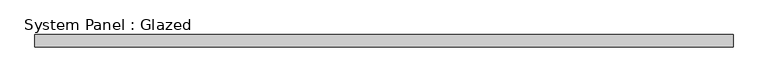
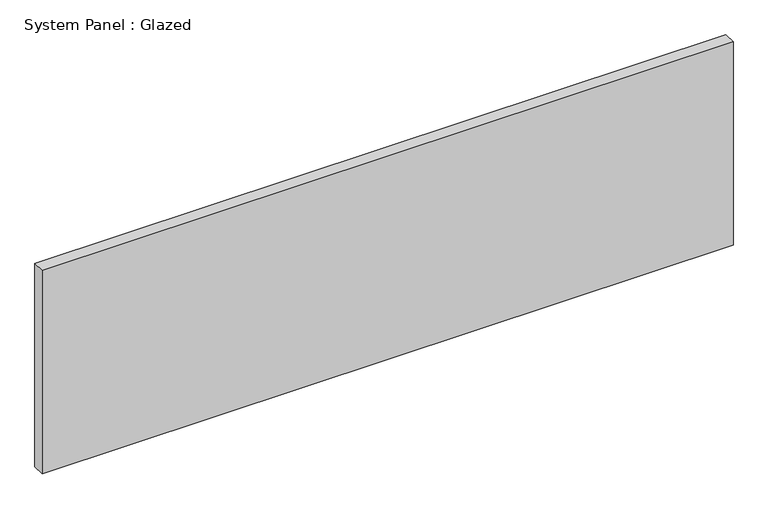
"""IFC4 building model written with IfcOpenShell, lengths in millimetres: plate geometry, System Panel : Glazed."""

from ifc_helpers import new_model, si_unit, origin, origin_with_axes, place, context, project, spatial, polyline, outline, extrude, source, transform, mapped, element, save


def system_panel_glazed_a826d7bb(model_context):
    return source(origin(), model_context, "Body", "SweptSolid", [
        extrude(outline(polyline([(714.375, 19.05), (-714.375, 19.05), (-714.375, 44.45), (714.375, 44.45), (714.375, 19.05)])), origin_with_axes(), (0.0, 0.0, 1.0), 444.5),
    ])


if __name__ == "__main__":
    model = new_model("IFC4")
    model_context = context("Model", 3, world=origin())
    ifc_project = project(units=[si_unit("LENGTHUNIT", "METRE", prefix="MILLI")], contexts=[model_context])
    site = spatial("IfcSite", under=ifc_project)
    building = spatial("IfcBuilding", under=site)
    placement = place(None, origin())
    system_panel_glazed_shape = system_panel_glazed_a826d7bb(model_context)
    element("IfcPlate", 1, ObjectType="System Panel : Glazed", at=placement, inside=building, context=model_context, shape_type="MappedRepresentation", body=[
        mapped(system_panel_glazed_shape, transform((0.0, 0.0, 0.0), x_axis=(1.0, 0.0, 0.0), y_axis=(0.0, 1.0, 0.0), z_axis=(0.0, 0.0, 1.0))),
    ])
    save(model, "model.ifc")

# Revit data of these elements
# Type "System Panel : Glazed"
#   Construction Type Id = "GSP4R"
#   Analytic Construction = "1/8 in Pilkington single glazing"
#   Visual Light Transmittance = 0.9
#   Solar Heat Gain Coefficient = 0.86
#   Heat Transfer Coefficient (U) = 1.18115 BTU/(h·ft²·°F)
#   Define Thermal Properties by = 1
# Element 1 (IfcPlate, "System Panel : Glazed")
#   Materials on its faces: "Glass"
# Materials
#   "Glass": class "Glass", colour RGB 0 128 192, transparency 0.75, Description = "Soda Lime Glass", Cost = 0
